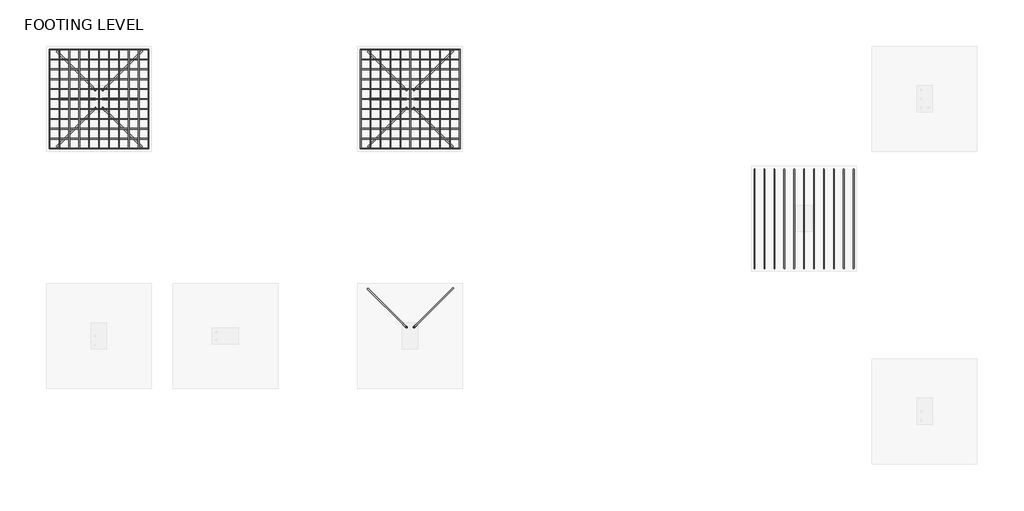
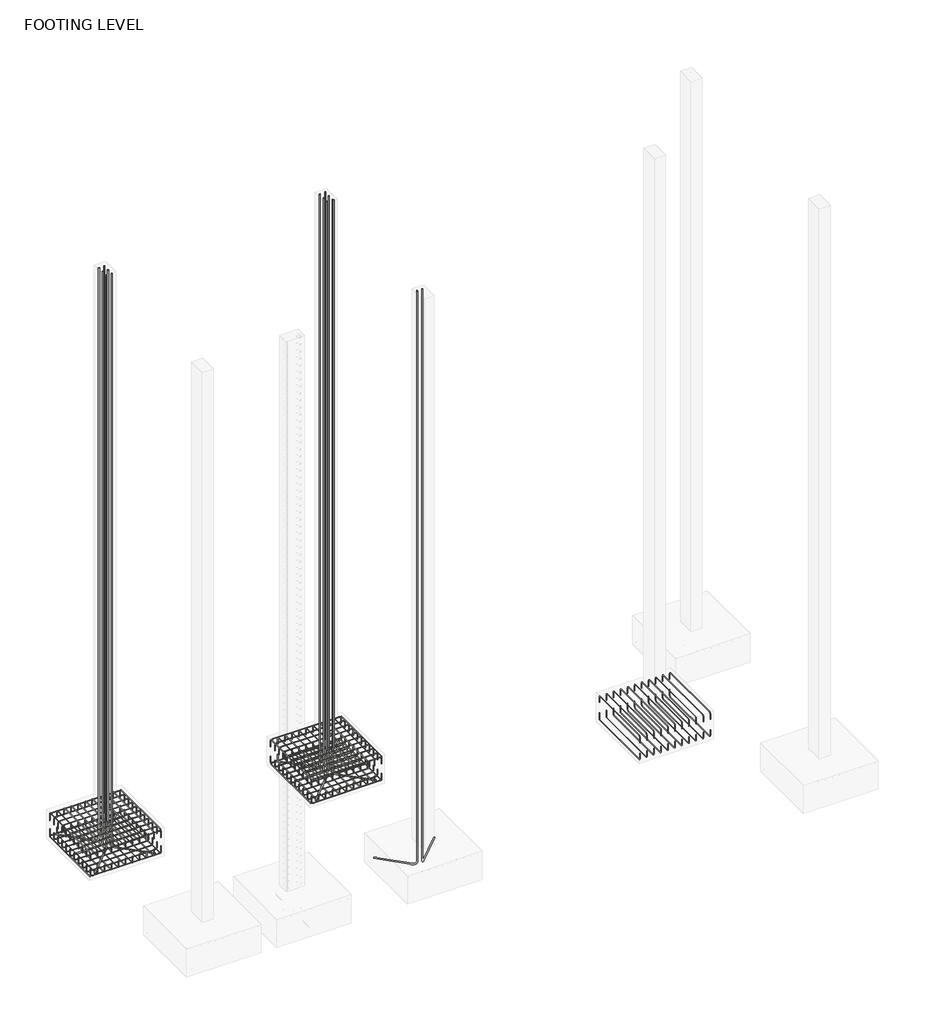
# One storey, part 9 of 10: 30 reinforcing bars.
"""IFC4 building model written with IfcOpenShell, lengths in millimetres."""

from ifc_helpers import new_model, si_unit, point, frame, origin, place, context, project, spatial, polyline, circle_curve, trimmed, segment, composite_curve, source, transform, mapped, element, save
from ifc_brep_helpers import swept_disk

model = new_model("IFC4")

# Units and contexts
model_context = context("Model", 3, world=origin())
ifc_project = project(units=[si_unit("LENGTHUNIT", "METRE", prefix="MILLI")], contexts=[model_context])

# Site, building, storey
site = spatial("IfcSite", under=ifc_project)
building = spatial("IfcBuilding", under=site)
storey = spatial("IfcBuildingStorey", under=building, Name="FOOTING LEVEL", Elevation=-1371.6)

# Reinforcing bars
placement = place(None, origin())
reinforcing_bar_shape = source(origin(), model_context, "Body", "SolidModel", [
    swept_disk(composite_curve([segment(polyline([(-9478.6043223, 13953.4953802, -1562.1), (-9478.6043223, 13953.4953802, -1447.8)]), True, "CONTINUOUS"), segment(trimmed(circle_curve(frame((-9478.6043223, 13920.1578802, -1447.8), z_axis=(1.0, 0.0, 0.0), x_axis=(0.0, 33.337499999999636, 0.0)), 33.3375), [point((-9478.6043223, 13953.4953802, -1447.8))], [point((-9478.6043223, 13920.1578802, -1414.4625))], True, "CARTESIAN"), True, "CONTINUOUS"), segment(polyline([(-9478.6043223, 13920.1578802, -1414.4625), (-9478.6043223, 12548.5578802, -1414.4625)]), True, "CONTINUOUS"), segment(trimmed(circle_curve(frame((-9478.6043223, 12548.5578802, -1447.8), z_axis=(1.0, 0.0, 0.0), x_axis=(0.0, 0.0, 33.337499999999864)), 33.3375), [point((-9478.6043223, 12548.5578802, -1414.4625))], [point((-9478.6043223, 12515.2203802, -1447.8))], True, "CARTESIAN"), True, "CONTINUOUS"), segment(polyline([(-9478.6043223, 12515.2203802, -1447.8), (-9478.6043223, 12515.2203802, -1562.1)]), True, "CONTINUOUS")], self_intersect=False), 4.7625),
])
element("IfcReinforcingBar", 1, at=placement, inside=storey, context=model_context, shape_type="MappedRepresentation", body=[
    mapped(reinforcing_bar_shape, transform((0.0, 0.0, 0.0), x_axis=(1.0, 0.0, 0.0), y_axis=(0.0, 1.0, 0.0), z_axis=(0.0, 0.0, 1.0))),
    mapped(reinforcing_bar_shape, transform((-143.8275, 0.0, 0.0), x_axis=(1.0, 0.0, 0.0), y_axis=(0.0, 1.0, 0.0), z_axis=(0.0, 0.0, 1.0))),
    mapped(reinforcing_bar_shape, transform((-287.655, 0.0, 0.0), x_axis=(1.0, 0.0, 0.0), y_axis=(0.0, 1.0, 0.0), z_axis=(0.0, 0.0, 1.0))),
    mapped(reinforcing_bar_shape, transform((-431.4825, 0.0, 0.0), x_axis=(1.0, 0.0, 0.0), y_axis=(0.0, 1.0, 0.0), z_axis=(0.0, 0.0, 1.0))),
    mapped(reinforcing_bar_shape, transform((-575.31, 0.0, 0.0), x_axis=(1.0, 0.0, 0.0), y_axis=(0.0, 1.0, 0.0), z_axis=(0.0, 0.0, 1.0))),
    mapped(reinforcing_bar_shape, transform((-719.1375, 0.0, 0.0), x_axis=(1.0, 0.0, 0.0), y_axis=(0.0, 1.0, 0.0), z_axis=(0.0, 0.0, 1.0))),
    mapped(reinforcing_bar_shape, transform((-862.965, 0.0, 0.0), x_axis=(1.0, 0.0, 0.0), y_axis=(0.0, 1.0, 0.0), z_axis=(0.0, 0.0, 1.0))),
    mapped(reinforcing_bar_shape, transform((-1006.7925, 0.0, 0.0), x_axis=(1.0, 0.0, 0.0), y_axis=(0.0, 1.0, 0.0), z_axis=(0.0, 0.0, 1.0))),
    mapped(reinforcing_bar_shape, transform((-1150.62, 0.0, 0.0), x_axis=(1.0, 0.0, 0.0), y_axis=(0.0, 1.0, 0.0), z_axis=(0.0, 0.0, 1.0))),
    mapped(reinforcing_bar_shape, transform((-1294.4475, 0.0, 0.0), x_axis=(1.0, 0.0, 0.0), y_axis=(0.0, 1.0, 0.0), z_axis=(0.0, 0.0, 1.0))),
    mapped(reinforcing_bar_shape, transform((-1438.275, 0.0, 0.0), x_axis=(1.0, 0.0, 0.0), y_axis=(0.0, 1.0, 0.0), z_axis=(0.0, 0.0, 1.0))),
])
reinforcing_bar_2_shape = source(origin(), model_context, "Body", "SolidModel", [
    swept_disk(composite_curve([segment(polyline([(-9478.6043223, 12515.2203802, -1790.7), (-9478.6043223, 12515.2203802, -1905.0)]), True, "CONTINUOUS"), segment(trimmed(circle_curve(frame((-9478.6043223, 12548.5578802, -1905.0), z_axis=(1.0, 0.0, 0.0), x_axis=(0.0, -33.337499999999636, 0.0)), 33.3375), [point((-9478.6043223, 12515.2203802, -1905.0))], [point((-9478.6043223, 12548.5578802, -1938.3375))], True, "CARTESIAN"), True, "CONTINUOUS"), segment(polyline([(-9478.6043223, 12548.5578802, -1938.3375), (-9478.6043223, 13920.1578802, -1938.3375)]), True, "CONTINUOUS"), segment(trimmed(circle_curve(frame((-9478.6043223, 13920.1578802, -1905.0), z_axis=(1.0, 0.0, 0.0), x_axis=(0.0, 0.0, -33.33750000000009)), 33.3375), [point((-9478.6043223, 13920.1578802, -1938.3375))], [point((-9478.6043223, 13953.4953802, -1905.0))], True, "CARTESIAN"), True, "CONTINUOUS"), segment(polyline([(-9478.6043223, 13953.4953802, -1905.0), (-9478.6043223, 13953.4953802, -1790.7)]), True, "CONTINUOUS")], self_intersect=False), 4.7625),
])
element("IfcReinforcingBar", 2, at=placement, inside=storey, context=model_context, shape_type="MappedRepresentation", body=[
    mapped(reinforcing_bar_2_shape, transform((0.0, 0.0, 0.0), x_axis=(1.0, 0.0, 0.0), y_axis=(0.0, 1.0, 0.0), z_axis=(0.0, 0.0, 1.0))),
    mapped(reinforcing_bar_2_shape, transform((-143.8275, 0.0, 0.0), x_axis=(1.0, 0.0, 0.0), y_axis=(0.0, 1.0, 0.0), z_axis=(0.0, 0.0, 1.0))),
    mapped(reinforcing_bar_2_shape, transform((-287.655, 0.0, 0.0), x_axis=(1.0, 0.0, 0.0), y_axis=(0.0, 1.0, 0.0), z_axis=(0.0, 0.0, 1.0))),
    mapped(reinforcing_bar_2_shape, transform((-431.4825, 0.0, 0.0), x_axis=(1.0, 0.0, 0.0), y_axis=(0.0, 1.0, 0.0), z_axis=(0.0, 0.0, 1.0))),
    mapped(reinforcing_bar_2_shape, transform((-575.31, 0.0, 0.0), x_axis=(1.0, 0.0, 0.0), y_axis=(0.0, 1.0, 0.0), z_axis=(0.0, 0.0, 1.0))),
    mapped(reinforcing_bar_2_shape, transform((-719.1375, 0.0, 0.0), x_axis=(1.0, 0.0, 0.0), y_axis=(0.0, 1.0, 0.0), z_axis=(0.0, 0.0, 1.0))),
    mapped(reinforcing_bar_2_shape, transform((-862.965, 0.0, 0.0), x_axis=(1.0, 0.0, 0.0), y_axis=(0.0, 1.0, 0.0), z_axis=(0.0, 0.0, 1.0))),
    mapped(reinforcing_bar_2_shape, transform((-1006.7925, 0.0, 0.0), x_axis=(1.0, 0.0, 0.0), y_axis=(0.0, 1.0, 0.0), z_axis=(0.0, 0.0, 1.0))),
    mapped(reinforcing_bar_2_shape, transform((-1150.62, 0.0, 0.0), x_axis=(1.0, 0.0, 0.0), y_axis=(0.0, 1.0, 0.0), z_axis=(0.0, 0.0, 1.0))),
    mapped(reinforcing_bar_2_shape, transform((-1294.4475, 0.0, 0.0), x_axis=(1.0, 0.0, 0.0), y_axis=(0.0, 1.0, 0.0), z_axis=(0.0, 0.0, 1.0))),
    mapped(reinforcing_bar_2_shape, transform((-1438.275, 0.0, 0.0), x_axis=(1.0, 0.0, 0.0), y_axis=(0.0, 1.0, 0.0), z_axis=(0.0, 0.0, 1.0))),
])
reinforcing_bar_3_shape = source(origin(), model_context, "Body", "SolidModel", [
    swept_disk(composite_curve([segment(polyline([(-13993.4543223, 13953.4953802, -1562.1), (-13993.4543223, 13953.4953802, -1447.8)]), True, "CONTINUOUS"), segment(trimmed(circle_curve(frame((-13993.4543223, 13920.1578802, -1447.8), z_axis=(1.0, 0.0, 0.0), x_axis=(0.0, 33.337499999999636, 0.0)), 33.3375), [point((-13993.4543223, 13953.4953802, -1447.8))], [point((-13993.4543223, 13920.1578802, -1414.4625))], True, "CARTESIAN"), True, "CONTINUOUS"), segment(polyline([(-13993.4543223, 13920.1578802, -1414.4625), (-13993.4543223, 12548.5578802, -1414.4625)]), True, "CONTINUOUS"), segment(trimmed(circle_curve(frame((-13993.4543223, 12548.5578802, -1447.8), z_axis=(1.0, 0.0, 0.0), x_axis=(0.0, 0.0, 33.337499999999864)), 33.3375), [point((-13993.4543223, 12548.5578802, -1414.4625))], [point((-13993.4543223, 12515.2203802, -1447.8))], True, "CARTESIAN"), True, "CONTINUOUS"), segment(polyline([(-13993.4543223, 12515.2203802, -1447.8), (-13993.4543223, 12515.2203802, -1562.1)]), True, "CONTINUOUS")], self_intersect=False), 4.7625),
])
element("IfcReinforcingBar", 3, at=placement, inside=storey, context=model_context, shape_type="MappedRepresentation", body=[
    mapped(reinforcing_bar_3_shape, transform((0.0, 0.0, 0.0), x_axis=(1.0, 0.0, 0.0), y_axis=(0.0, 1.0, 0.0), z_axis=(0.0, 0.0, 1.0))),
    mapped(reinforcing_bar_3_shape, transform((-143.8275, 0.0, 0.0), x_axis=(1.0, 0.0, 0.0), y_axis=(0.0, 1.0, 0.0), z_axis=(0.0, 0.0, 1.0))),
    mapped(reinforcing_bar_3_shape, transform((-287.655, 0.0, 0.0), x_axis=(1.0, 0.0, 0.0), y_axis=(0.0, 1.0, 0.0), z_axis=(0.0, 0.0, 1.0))),
    mapped(reinforcing_bar_3_shape, transform((-431.4825, 0.0, 0.0), x_axis=(1.0, 0.0, 0.0), y_axis=(0.0, 1.0, 0.0), z_axis=(0.0, 0.0, 1.0))),
    mapped(reinforcing_bar_3_shape, transform((-575.31, 0.0, 0.0), x_axis=(1.0, 0.0, 0.0), y_axis=(0.0, 1.0, 0.0), z_axis=(0.0, 0.0, 1.0))),
    mapped(reinforcing_bar_3_shape, transform((-719.1375, 0.0, 0.0), x_axis=(1.0, 0.0, 0.0), y_axis=(0.0, 1.0, 0.0), z_axis=(0.0, 0.0, 1.0))),
    mapped(reinforcing_bar_3_shape, transform((-862.965, 0.0, 0.0), x_axis=(1.0, 0.0, 0.0), y_axis=(0.0, 1.0, 0.0), z_axis=(0.0, 0.0, 1.0))),
    mapped(reinforcing_bar_3_shape, transform((-1006.7925, 0.0, 0.0), x_axis=(1.0, 0.0, 0.0), y_axis=(0.0, 1.0, 0.0), z_axis=(0.0, 0.0, 1.0))),
    mapped(reinforcing_bar_3_shape, transform((-1150.62, 0.0, 0.0), x_axis=(1.0, 0.0, 0.0), y_axis=(0.0, 1.0, 0.0), z_axis=(0.0, 0.0, 1.0))),
    mapped(reinforcing_bar_3_shape, transform((-1294.4475, 0.0, 0.0), x_axis=(1.0, 0.0, 0.0), y_axis=(0.0, 1.0, 0.0), z_axis=(0.0, 0.0, 1.0))),
    mapped(reinforcing_bar_3_shape, transform((-1438.275, 0.0, 0.0), x_axis=(1.0, 0.0, 0.0), y_axis=(0.0, 1.0, 0.0), z_axis=(0.0, 0.0, 1.0))),
])
reinforcing_bar_4_shape = source(origin(), model_context, "Body", "SolidModel", [
    swept_disk(composite_curve([segment(polyline([(-13993.4543223, 12515.2203802, -1790.7), (-13993.4543223, 12515.2203802, -1905.0)]), True, "CONTINUOUS"), segment(trimmed(circle_curve(frame((-13993.4543223, 12548.5578802, -1905.0), z_axis=(1.0, 0.0, 0.0), x_axis=(0.0, -33.337499999999636, 0.0)), 33.3375), [point((-13993.4543223, 12515.2203802, -1905.0))], [point((-13993.4543223, 12548.5578802, -1938.3375))], True, "CARTESIAN"), True, "CONTINUOUS"), segment(polyline([(-13993.4543223, 12548.5578802, -1938.3375), (-13993.4543223, 13920.1578802, -1938.3375)]), True, "CONTINUOUS"), segment(trimmed(circle_curve(frame((-13993.4543223, 13920.1578802, -1905.0), z_axis=(1.0, 0.0, 0.0), x_axis=(0.0, 0.0, -33.33750000000009)), 33.3375), [point((-13993.4543223, 13920.1578802, -1938.3375))], [point((-13993.4543223, 13953.4953802, -1905.0))], True, "CARTESIAN"), True, "CONTINUOUS"), segment(polyline([(-13993.4543223, 13953.4953802, -1905.0), (-13993.4543223, 13953.4953802, -1790.7)]), True, "CONTINUOUS")], self_intersect=False), 4.7625),
])
element("IfcReinforcingBar", 4, at=placement, inside=storey, context=model_context, shape_type="MappedRepresentation", body=[
    mapped(reinforcing_bar_4_shape, transform((0.0, 0.0, 0.0), x_axis=(1.0, 0.0, 0.0), y_axis=(0.0, 1.0, 0.0), z_axis=(0.0, 0.0, 1.0))),
    mapped(reinforcing_bar_4_shape, transform((-143.8275, 0.0, 0.0), x_axis=(1.0, 0.0, 0.0), y_axis=(0.0, 1.0, 0.0), z_axis=(0.0, 0.0, 1.0))),
    mapped(reinforcing_bar_4_shape, transform((-287.655, 0.0, 0.0), x_axis=(1.0, 0.0, 0.0), y_axis=(0.0, 1.0, 0.0), z_axis=(0.0, 0.0, 1.0))),
    mapped(reinforcing_bar_4_shape, transform((-431.4825, 0.0, 0.0), x_axis=(1.0, 0.0, 0.0), y_axis=(0.0, 1.0, 0.0), z_axis=(0.0, 0.0, 1.0))),
    mapped(reinforcing_bar_4_shape, transform((-575.31, 0.0, 0.0), x_axis=(1.0, 0.0, 0.0), y_axis=(0.0, 1.0, 0.0), z_axis=(0.0, 0.0, 1.0))),
    mapped(reinforcing_bar_4_shape, transform((-719.1375, 0.0, 0.0), x_axis=(1.0, 0.0, 0.0), y_axis=(0.0, 1.0, 0.0), z_axis=(0.0, 0.0, 1.0))),
    mapped(reinforcing_bar_4_shape, transform((-862.965, 0.0, 0.0), x_axis=(1.0, 0.0, 0.0), y_axis=(0.0, 1.0, 0.0), z_axis=(0.0, 0.0, 1.0))),
    mapped(reinforcing_bar_4_shape, transform((-1006.7925, 0.0, 0.0), x_axis=(1.0, 0.0, 0.0), y_axis=(0.0, 1.0, 0.0), z_axis=(0.0, 0.0, 1.0))),
    mapped(reinforcing_bar_4_shape, transform((-1150.62, 0.0, 0.0), x_axis=(1.0, 0.0, 0.0), y_axis=(0.0, 1.0, 0.0), z_axis=(0.0, 0.0, 1.0))),
    mapped(reinforcing_bar_4_shape, transform((-1294.4475, 0.0, 0.0), x_axis=(1.0, 0.0, 0.0), y_axis=(0.0, 1.0, 0.0), z_axis=(0.0, 0.0, 1.0))),
    mapped(reinforcing_bar_4_shape, transform((-1438.275, 0.0, 0.0), x_axis=(1.0, 0.0, 0.0), y_axis=(0.0, 1.0, 0.0), z_axis=(0.0, 0.0, 1.0))),
])
reinforcing_bar_5_shape = source(origin(), model_context, "Body", "SolidModel", [
    swept_disk(composite_curve([segment(polyline([(-15431.7293223, 12515.2203802, -1770.864029), (-15431.7293223, 12515.2203802, -1885.164029)]), True, "CONTINUOUS"), segment(trimmed(circle_curve(frame((-15398.3918223, 12515.2203802, -1885.164029), z_axis=(0.0, -1.0, 0.0), x_axis=(-33.337499999999636, 0.0, 0.0)), 33.3375), [point((-15431.7293223, 12515.2203802, -1885.164029))], [point((-15398.3918223, 12515.2203802, -1918.501529))], True, "CARTESIAN"), True, "CONTINUOUS"), segment(polyline([(-15398.3918223, 12515.2203802, -1918.501529), (-14026.7918223, 12515.2203802, -1918.501529)]), True, "CONTINUOUS"), segment(trimmed(circle_curve(frame((-14026.7918223, 12515.2203802, -1885.164029), z_axis=(0.0, -1.0, 0.0), x_axis=(0.0, 0.0, -33.337499999999864)), 33.3375), [point((-14026.7918223, 12515.2203802, -1918.501529))], [point((-13993.4543223, 12515.2203802, -1885.164029))], True, "CARTESIAN"), True, "CONTINUOUS"), segment(polyline([(-13993.4543223, 12515.2203802, -1885.164029), (-13993.4543223, 12515.2203802, -1770.864029)]), True, "CONTINUOUS")], self_intersect=False), 4.7625),
])
element("IfcReinforcingBar", 5, at=placement, inside=storey, context=model_context, shape_type="MappedRepresentation", body=[
    mapped(reinforcing_bar_5_shape, transform((0.0, 0.0, 0.0), x_axis=(1.0, 0.0, 0.0), y_axis=(0.0, 1.0, 0.0), z_axis=(0.0, 0.0, 1.0))),
    mapped(reinforcing_bar_5_shape, transform((0.0, 143.8275, 0.0), x_axis=(1.0, 0.0, 0.0), y_axis=(0.0, 1.0, 0.0), z_axis=(0.0, 0.0, 1.0))),
    mapped(reinforcing_bar_5_shape, transform((0.0, 287.655, 0.0), x_axis=(1.0, 0.0, 0.0), y_axis=(0.0, 1.0, 0.0), z_axis=(0.0, 0.0, 1.0))),
    mapped(reinforcing_bar_5_shape, transform((0.0, 431.4825, 0.0), x_axis=(1.0, 0.0, 0.0), y_axis=(0.0, 1.0, 0.0), z_axis=(0.0, 0.0, 1.0))),
    mapped(reinforcing_bar_5_shape, transform((0.0, 575.31, 0.0), x_axis=(1.0, 0.0, 0.0), y_axis=(0.0, 1.0, 0.0), z_axis=(0.0, 0.0, 1.0))),
    mapped(reinforcing_bar_5_shape, transform((0.0, 719.1375, 0.0), x_axis=(1.0, 0.0, 0.0), y_axis=(0.0, 1.0, 0.0), z_axis=(0.0, 0.0, 1.0))),
    mapped(reinforcing_bar_5_shape, transform((0.0, 862.965, 0.0), x_axis=(1.0, 0.0, 0.0), y_axis=(0.0, 1.0, 0.0), z_axis=(0.0, 0.0, 1.0))),
    mapped(reinforcing_bar_5_shape, transform((0.0, 1006.7925, 0.0), x_axis=(1.0, 0.0, 0.0), y_axis=(0.0, 1.0, 0.0), z_axis=(0.0, 0.0, 1.0))),
    mapped(reinforcing_bar_5_shape, transform((0.0, 1150.62, 0.0), x_axis=(1.0, 0.0, 0.0), y_axis=(0.0, 1.0, 0.0), z_axis=(0.0, 0.0, 1.0))),
    mapped(reinforcing_bar_5_shape, transform((0.0, 1294.4475, 0.0), x_axis=(1.0, 0.0, 0.0), y_axis=(0.0, 1.0, 0.0), z_axis=(0.0, 0.0, 1.0))),
    mapped(reinforcing_bar_5_shape, transform((0.0, 1438.275, 0.0), x_axis=(1.0, 0.0, 0.0), y_axis=(0.0, 1.0, 0.0), z_axis=(0.0, 0.0, 1.0))),
])
reinforcing_bar_6_shape = source(origin(), model_context, "Body", "SolidModel", [
    swept_disk(composite_curve([segment(polyline([(-15431.7293223, 13953.4953802, -1586.5406765), (-15431.7293223, 13953.4953802, -1472.2406765)]), True, "CONTINUOUS"), segment(trimmed(circle_curve(frame((-15398.3918223, 13953.4953802, -1472.2406765), z_axis=(0.0, 1.0, 0.0), x_axis=(-33.337499999999636, 0.0, 0.0)), 33.3375), [point((-15431.7293223, 13953.4953802, -1472.2406765))], [point((-15398.3918223, 13953.4953802, -1438.9031765))], True, "CARTESIAN"), True, "CONTINUOUS"), segment(polyline([(-15398.3918223, 13953.4953802, -1438.9031765), (-14026.7918223, 13953.4953802, -1438.9031765)]), True, "CONTINUOUS"), segment(trimmed(circle_curve(frame((-14026.7918223, 13953.4953802, -1472.2406765), z_axis=(0.0, 1.0, 0.0), x_axis=(0.0, 0.0, 33.33750000000009)), 33.3375), [point((-14026.7918223, 13953.4953802, -1438.9031765))], [point((-13993.4543223, 13953.4953802, -1472.2406765))], True, "CARTESIAN"), True, "CONTINUOUS"), segment(polyline([(-13993.4543223, 13953.4953802, -1472.2406765), (-13993.4543223, 13953.4953802, -1586.5406765)]), True, "CONTINUOUS")], self_intersect=False), 4.7625),
])
element("IfcReinforcingBar", 6, at=placement, inside=storey, context=model_context, shape_type="MappedRepresentation", body=[
    mapped(reinforcing_bar_6_shape, transform((0.0, 0.0, 0.0), x_axis=(1.0, 0.0, 0.0), y_axis=(0.0, 1.0, 0.0), z_axis=(0.0, 0.0, 1.0))),
    mapped(reinforcing_bar_6_shape, transform((0.0, -143.8275, 0.0), x_axis=(1.0, 0.0, 0.0), y_axis=(0.0, 1.0, 0.0), z_axis=(0.0, 0.0, 1.0))),
    mapped(reinforcing_bar_6_shape, transform((0.0, -287.655, 0.0), x_axis=(1.0, 0.0, 0.0), y_axis=(0.0, 1.0, 0.0), z_axis=(0.0, 0.0, 1.0))),
    mapped(reinforcing_bar_6_shape, transform((0.0, -431.4825, 0.0), x_axis=(1.0, 0.0, 0.0), y_axis=(0.0, 1.0, 0.0), z_axis=(0.0, 0.0, 1.0))),
    mapped(reinforcing_bar_6_shape, transform((0.0, -575.31, 0.0), x_axis=(1.0, 0.0, 0.0), y_axis=(0.0, 1.0, 0.0), z_axis=(0.0, 0.0, 1.0))),
    mapped(reinforcing_bar_6_shape, transform((0.0, -719.1375, 0.0), x_axis=(1.0, 0.0, 0.0), y_axis=(0.0, 1.0, 0.0), z_axis=(0.0, 0.0, 1.0))),
    mapped(reinforcing_bar_6_shape, transform((0.0, -862.965, 0.0), x_axis=(1.0, 0.0, 0.0), y_axis=(0.0, 1.0, 0.0), z_axis=(0.0, 0.0, 1.0))),
    mapped(reinforcing_bar_6_shape, transform((0.0, -1006.7925, 0.0), x_axis=(1.0, 0.0, 0.0), y_axis=(0.0, 1.0, 0.0), z_axis=(0.0, 0.0, 1.0))),
    mapped(reinforcing_bar_6_shape, transform((0.0, -1150.62, 0.0), x_axis=(1.0, 0.0, 0.0), y_axis=(0.0, 1.0, 0.0), z_axis=(0.0, 0.0, 1.0))),
    mapped(reinforcing_bar_6_shape, transform((0.0, -1294.4475, 0.0), x_axis=(1.0, 0.0, 0.0), y_axis=(0.0, 1.0, 0.0), z_axis=(0.0, 0.0, 1.0))),
    mapped(reinforcing_bar_6_shape, transform((0.0, -1438.275, 0.0), x_axis=(1.0, 0.0, 0.0), y_axis=(0.0, 1.0, 0.0), z_axis=(0.0, 0.0, 1.0))),
])
reinforcing_bar_7_shape = source(origin(), model_context, "Body", "SolidModel", [
    swept_disk(composite_curve([segment(polyline([(-3763.6043223, 12216.291297, -1562.1), (-3763.6043223, 12216.291297, -1447.8)]), True, "CONTINUOUS"), segment(trimmed(circle_curve(frame((-3763.6043223, 12182.953797, -1447.8), z_axis=(1.0, 0.0, 0.0), x_axis=(0.0, 33.337499999999636, 0.0)), 33.3375), [point((-3763.6043223, 12216.291297, -1447.8))], [point((-3763.6043223, 12182.953797, -1414.4625))], True, "CARTESIAN"), True, "CONTINUOUS"), segment(polyline([(-3763.6043223, 12182.953797, -1414.4625), (-3763.6043223, 10811.353797, -1414.4625)]), True, "CONTINUOUS"), segment(trimmed(circle_curve(frame((-3763.6043223, 10811.353797, -1447.8), z_axis=(1.0, 0.0, 0.0), x_axis=(0.0, 0.0, 33.337499999999864)), 33.3375), [point((-3763.6043223, 10811.353797, -1414.4625))], [point((-3763.6043223, 10778.016297, -1447.8))], True, "CARTESIAN"), True, "CONTINUOUS"), segment(polyline([(-3763.6043223, 10778.016297, -1447.8), (-3763.6043223, 10778.016297, -1562.1)]), True, "CONTINUOUS")], self_intersect=False), 4.7625),
])
element("IfcReinforcingBar", 7, at=placement, inside=storey, context=model_context, shape_type="MappedRepresentation", body=[
    mapped(reinforcing_bar_7_shape, transform((0.0, 0.0, 0.0), x_axis=(1.0, 0.0, 0.0), y_axis=(0.0, 1.0, 0.0), z_axis=(0.0, 0.0, 1.0))),
    mapped(reinforcing_bar_7_shape, transform((-143.8275, 0.0, 0.0), x_axis=(1.0, 0.0, 0.0), y_axis=(0.0, 1.0, 0.0), z_axis=(0.0, 0.0, 1.0))),
    mapped(reinforcing_bar_7_shape, transform((-287.655, 0.0, 0.0), x_axis=(1.0, 0.0, 0.0), y_axis=(0.0, 1.0, 0.0), z_axis=(0.0, 0.0, 1.0))),
    mapped(reinforcing_bar_7_shape, transform((-431.4825, 0.0, 0.0), x_axis=(1.0, 0.0, 0.0), y_axis=(0.0, 1.0, 0.0), z_axis=(0.0, 0.0, 1.0))),
    mapped(reinforcing_bar_7_shape, transform((-575.31, 0.0, 0.0), x_axis=(1.0, 0.0, 0.0), y_axis=(0.0, 1.0, 0.0), z_axis=(0.0, 0.0, 1.0))),
    mapped(reinforcing_bar_7_shape, transform((-719.1375, 0.0, 0.0), x_axis=(1.0, 0.0, 0.0), y_axis=(0.0, 1.0, 0.0), z_axis=(0.0, 0.0, 1.0))),
    mapped(reinforcing_bar_7_shape, transform((-862.965, 0.0, 0.0), x_axis=(1.0, 0.0, 0.0), y_axis=(0.0, 1.0, 0.0), z_axis=(0.0, 0.0, 1.0))),
    mapped(reinforcing_bar_7_shape, transform((-1006.7925, 0.0, 0.0), x_axis=(1.0, 0.0, 0.0), y_axis=(0.0, 1.0, 0.0), z_axis=(0.0, 0.0, 1.0))),
    mapped(reinforcing_bar_7_shape, transform((-1150.62, 0.0, 0.0), x_axis=(1.0, 0.0, 0.0), y_axis=(0.0, 1.0, 0.0), z_axis=(0.0, 0.0, 1.0))),
    mapped(reinforcing_bar_7_shape, transform((-1294.4475, 0.0, 0.0), x_axis=(1.0, 0.0, 0.0), y_axis=(0.0, 1.0, 0.0), z_axis=(0.0, 0.0, 1.0))),
    mapped(reinforcing_bar_7_shape, transform((-1438.275, 0.0, 0.0), x_axis=(1.0, 0.0, 0.0), y_axis=(0.0, 1.0, 0.0), z_axis=(0.0, 0.0, 1.0))),
])
reinforcing_bar_8_shape = source(origin(), model_context, "Body", "SolidModel", [
    swept_disk(composite_curve([segment(polyline([(-3763.6043223, 10778.016297, -1790.7), (-3763.6043223, 10778.016297, -1905.0)]), True, "CONTINUOUS"), segment(trimmed(circle_curve(frame((-3763.6043223, 10811.353797, -1905.0), z_axis=(1.0, 0.0, 0.0), x_axis=(0.0, -33.337499999999636, 0.0)), 33.3375), [point((-3763.6043223, 10778.016297, -1905.0))], [point((-3763.6043223, 10811.353797, -1938.3375))], True, "CARTESIAN"), True, "CONTINUOUS"), segment(polyline([(-3763.6043223, 10811.353797, -1938.3375), (-3763.6043223, 12182.953797, -1938.3375)]), True, "CONTINUOUS"), segment(trimmed(circle_curve(frame((-3763.6043223, 12182.953797, -1905.0), z_axis=(1.0, 0.0, 0.0), x_axis=(0.0, 0.0, -33.33750000000009)), 33.3375), [point((-3763.6043223, 12182.953797, -1938.3375))], [point((-3763.6043223, 12216.291297, -1905.0))], True, "CARTESIAN"), True, "CONTINUOUS"), segment(polyline([(-3763.6043223, 12216.291297, -1905.0), (-3763.6043223, 12216.291297, -1790.7)]), True, "CONTINUOUS")], self_intersect=False), 4.7625),
])
element("IfcReinforcingBar", 8, at=placement, inside=storey, context=model_context, shape_type="MappedRepresentation", body=[
    mapped(reinforcing_bar_8_shape, transform((0.0, 0.0, 0.0), x_axis=(1.0, 0.0, 0.0), y_axis=(0.0, 1.0, 0.0), z_axis=(0.0, 0.0, 1.0))),
    mapped(reinforcing_bar_8_shape, transform((-143.8275, 0.0, 0.0), x_axis=(1.0, 0.0, 0.0), y_axis=(0.0, 1.0, 0.0), z_axis=(0.0, 0.0, 1.0))),
    mapped(reinforcing_bar_8_shape, transform((-287.655, 0.0, 0.0), x_axis=(1.0, 0.0, 0.0), y_axis=(0.0, 1.0, 0.0), z_axis=(0.0, 0.0, 1.0))),
    mapped(reinforcing_bar_8_shape, transform((-431.4825, 0.0, 0.0), x_axis=(1.0, 0.0, 0.0), y_axis=(0.0, 1.0, 0.0), z_axis=(0.0, 0.0, 1.0))),
    mapped(reinforcing_bar_8_shape, transform((-575.31, 0.0, 0.0), x_axis=(1.0, 0.0, 0.0), y_axis=(0.0, 1.0, 0.0), z_axis=(0.0, 0.0, 1.0))),
    mapped(reinforcing_bar_8_shape, transform((-719.1375, 0.0, 0.0), x_axis=(1.0, 0.0, 0.0), y_axis=(0.0, 1.0, 0.0), z_axis=(0.0, 0.0, 1.0))),
    mapped(reinforcing_bar_8_shape, transform((-862.965, 0.0, 0.0), x_axis=(1.0, 0.0, 0.0), y_axis=(0.0, 1.0, 0.0), z_axis=(0.0, 0.0, 1.0))),
    mapped(reinforcing_bar_8_shape, transform((-1006.7925, 0.0, 0.0), x_axis=(1.0, 0.0, 0.0), y_axis=(0.0, 1.0, 0.0), z_axis=(0.0, 0.0, 1.0))),
    mapped(reinforcing_bar_8_shape, transform((-1150.62, 0.0, 0.0), x_axis=(1.0, 0.0, 0.0), y_axis=(0.0, 1.0, 0.0), z_axis=(0.0, 0.0, 1.0))),
    mapped(reinforcing_bar_8_shape, transform((-1294.4475, 0.0, 0.0), x_axis=(1.0, 0.0, 0.0), y_axis=(0.0, 1.0, 0.0), z_axis=(0.0, 0.0, 1.0))),
    mapped(reinforcing_bar_8_shape, transform((-1438.275, 0.0, 0.0), x_axis=(1.0, 0.0, 0.0), y_axis=(0.0, 1.0, 0.0), z_axis=(0.0, 0.0, 1.0))),
])
element("IfcReinforcingBar", 9, at=placement, inside=storey, context=model_context, shape_type="SolidModel", body=[
    swept_disk(composite_curve([segment(polyline([(-14658.2316302, 13364.9180723, -1333.5), (-14658.2316302, 13364.9180723, 10477.5)]), True, "CONTINUOUS")], self_intersect=False), 9.525),
])
element("IfcReinforcingBar", 10, at=placement, inside=storey, context=model_context, shape_type="SolidModel", body=[
    swept_disk(composite_curve([segment(polyline([(-14766.9520144, 13103.7976881, -1333.5), (-14766.9520144, 13103.7976881, 10477.5)]), True, "CONTINUOUS")], self_intersect=False), 9.525),
])
element("IfcReinforcingBar", 11, at=placement, inside=storey, context=model_context, shape_type="SolidModel", body=[
    swept_disk(composite_curve([segment(polyline([(-14658.2316302, 13103.7976881, -1333.5), (-14658.2316302, 13103.7976881, 10477.5)]), True, "CONTINUOUS")], self_intersect=False), 9.525),
])
element("IfcReinforcingBar", 12, at=placement, inside=storey, context=model_context, shape_type="SolidModel", body=[
    swept_disk(composite_curve([segment(polyline([(-15328.6277703, 13926.5938282, -1910.4342608), (-14814.0983591, 13412.0644169, -1910.4342608)]), True, "CONTINUOUS"), segment(trimmed(circle_curve(frame((-14814.0983591, 13412.0644169, -1843.7592608), z_axis=(-0.7071067811865736, -0.7071067811865216, 0.0), x_axis=(0.0, 0.0, -66.67499999999995)), 66.675), [point((-14814.0983591, 13412.0644169, -1910.4342608))], [point((-14766.9520144, 13364.9180723, -1843.7592608))], True, "CARTESIAN"), True, "CONTINUOUS"), segment(polyline([(-14766.9520144, 13364.9180723, -1843.7592608), (-14766.9520144, 13364.9180723, 10477.5)]), True, "CONTINUOUS")], self_intersect=False), 9.525),
])
element("IfcReinforcingBar", 13, at=placement, inside=storey, context=model_context, shape_type="SolidModel", body=[
    swept_disk(composite_curve([segment(polyline([(-14088.5374965, 13934.612206, -1910.4342608), (-14611.0852856, 13412.0644169, -1910.4342608)]), True, "CONTINUOUS"), segment(trimmed(circle_curve(frame((-14611.0852856, 13412.0644169, -1843.7592608), z_axis=(-0.7071067811865712, 0.7071067811865238, 0.0), x_axis=(0.0, 0.0, -66.67499999999995)), 66.675), [point((-14611.0852856, 13412.0644169, -1910.4342608))], [point((-14658.2316302, 13364.9180723, -1843.7592608))], True, "CARTESIAN"), True, "CONTINUOUS"), segment(polyline([(-14658.2316302, 13364.9180723, -1843.7592608), (-14658.2316302, 13364.9180723, 10477.5)]), True, "CONTINUOUS")], self_intersect=False), 9.525),
])
element("IfcReinforcingBar", 14, at=placement, inside=storey, context=model_context, shape_type="SolidModel", body=[
    swept_disk(composite_curve([segment(polyline([(-15325.6711349, 12545.0785676, -1910.4342608), (-14814.0983591, 13056.6513434, -1910.4342608)]), True, "CONTINUOUS"), segment(trimmed(circle_curve(frame((-14814.0983591, 13056.6513434, -1843.7592608), z_axis=(0.707106781186576, -0.7071067811865192, 0.0), x_axis=(0.0, 0.0, -66.67499999999995)), 66.675), [point((-14814.0983591, 13056.6513434, -1910.4342608))], [point((-14766.9520144, 13103.7976881, -1843.7592608))], True, "CARTESIAN"), True, "CONTINUOUS"), segment(polyline([(-14766.9520144, 13103.7976881, -1843.7592608), (-14766.9520144, 13103.7976881, 10477.5)]), True, "CONTINUOUS")], self_intersect=False), 9.525),
])
element("IfcReinforcingBar", 15, at=placement, inside=storey, context=model_context, shape_type="SolidModel", body=[
    swept_disk(composite_curve([segment(polyline([(-14094.0528099, 12539.6188678, -1910.4342608), (-14611.0852856, 13056.6513434, -1910.4342608)]), True, "CONTINUOUS"), segment(trimmed(circle_curve(frame((-14611.0852856, 13056.6513434, -1843.7592608), z_axis=(0.7071067811865689, 0.7071067811865261, 0.0), x_axis=(0.0, 0.0, -66.67499999999995)), 66.675), [point((-14611.0852856, 13056.6513434, -1910.4342608))], [point((-14658.2316302, 13103.7976881, -1843.7592608))], True, "CARTESIAN"), True, "CONTINUOUS"), segment(polyline([(-14658.2316302, 13103.7976881, -1843.7592608), (-14658.2316302, 13103.7976881, 10477.5)]), True, "CONTINUOUS")], self_intersect=False), 9.525),
])
element("IfcReinforcingBar", 16, at=placement, inside=storey, context=model_context, shape_type="SolidModel", body=[
    swept_disk(composite_curve([segment(polyline([(-15305.1818909, 13234.3578802, -1910.4342608), (-14833.6270144, 13234.3578802, -1910.4342608)]), True, "CONTINUOUS"), segment(trimmed(circle_curve(frame((-14833.6270144, 13234.3578802, -1843.7592608), z_axis=(0.0, -1.0, 0.0), x_axis=(0.0, 0.0, -66.67499999999995)), 66.675), [point((-14833.6270144, 13234.3578802, -1910.4342608))], [point((-14766.9520144, 13234.3578802, -1843.7592608))], True, "CARTESIAN"), True, "CONTINUOUS"), segment(polyline([(-14766.9520144, 13234.3578802, -1843.7592608), (-14766.9520144, 13234.3578802, 10477.5)]), True, "CONTINUOUS")], self_intersect=False), 9.525),
])
element("IfcReinforcingBar", 17, at=placement, inside=storey, context=model_context, shape_type="SolidModel", body=[
    swept_disk(composite_curve([segment(polyline([(-10130.6816302, 13377.6180723, -1346.2), (-10130.6816302, 13377.6180723, 10490.2)]), True, "CONTINUOUS")], self_intersect=False), 9.525),
])
element("IfcReinforcingBar", 18, at=placement, inside=storey, context=model_context, shape_type="SolidModel", body=[
    swept_disk(composite_curve([segment(polyline([(-10264.8020144, 13091.0976881, -1346.2), (-10264.8020144, 13091.0976881, 10490.2)]), True, "CONTINUOUS")], self_intersect=False), 9.525),
])
element("IfcReinforcingBar", 19, at=placement, inside=storey, context=model_context, shape_type="SolidModel", body=[
    swept_disk(composite_curve([segment(polyline([(-10130.6816302, 13091.0976881, -1346.2), (-10130.6816302, 13091.0976881, 10490.2)]), True, "CONTINUOUS")], self_intersect=False), 9.525),
])
element("IfcReinforcingBar", 20, at=placement, inside=storey, context=model_context, shape_type="SolidModel", body=[
    swept_disk(composite_curve([segment(polyline([(-10813.7777703, 13926.5938282, -1910.4342608), (-10299.2483591, 13412.0644169, -1910.4342608)]), True, "CONTINUOUS"), segment(trimmed(circle_curve(frame((-10299.2483591, 13412.0644169, -1843.7592608), z_axis=(-0.7071067811865736, -0.7071067811865216, 0.0), x_axis=(0.0, 0.0, -66.67499999999995)), 66.675), [point((-10299.2483591, 13412.0644169, -1910.4342608))], [point((-10252.1020144, 13364.9180723, -1843.7592608))], True, "CARTESIAN"), True, "CONTINUOUS"), segment(polyline([(-10252.1020144, 13364.9180723, -1843.7592608), (-10252.1020144, 13364.9180723, 10490.2)]), True, "CONTINUOUS")], self_intersect=False), 9.525),
])
element("IfcReinforcingBar", 21, at=placement, inside=storey, context=model_context, shape_type="SolidModel", body=[
    swept_disk(composite_curve([segment(polyline([(-9573.6874965, 13934.612206, -1910.4342608), (-10096.2352856, 13412.0644169, -1910.4342608)]), True, "CONTINUOUS"), segment(trimmed(circle_curve(frame((-10096.2352856, 13412.0644169, -1843.7592608), z_axis=(-0.7071067811865712, 0.7071067811865238, 0.0), x_axis=(0.0, 0.0, -66.67499999999995)), 66.675), [point((-10096.2352856, 13412.0644169, -1910.4342608))], [point((-10143.3816302, 13364.9180723, -1843.7592608))], True, "CARTESIAN"), True, "CONTINUOUS"), segment(polyline([(-10143.3816302, 13364.9180723, -1843.7592608), (-10143.3816302, 13364.9180723, 10490.2)]), True, "CONTINUOUS")], self_intersect=False), 9.525),
])
element("IfcReinforcingBar", 22, at=placement, inside=storey, context=model_context, shape_type="SolidModel", body=[
    swept_disk(composite_curve([segment(polyline([(-10810.8211349, 12545.0785676, -1910.4342608), (-10299.2483591, 13056.6513434, -1910.4342608)]), True, "CONTINUOUS"), segment(trimmed(circle_curve(frame((-10299.2483591, 13056.6513434, -1843.7592608), z_axis=(0.707106781186576, -0.7071067811865192, 0.0), x_axis=(0.0, 0.0, -66.67499999999995)), 66.675), [point((-10299.2483591, 13056.6513434, -1910.4342608))], [point((-10252.1020144, 13103.7976881, -1843.7592608))], True, "CARTESIAN"), True, "CONTINUOUS"), segment(polyline([(-10252.1020144, 13103.7976881, -1843.7592608), (-10252.1020144, 13103.7976881, 10490.2)]), True, "CONTINUOUS")], self_intersect=False), 9.525),
])
element("IfcReinforcingBar", 23, at=placement, inside=storey, context=model_context, shape_type="SolidModel", body=[
    swept_disk(composite_curve([segment(polyline([(-9579.2028099, 12539.6188678, -1910.4342608), (-10096.2352856, 13056.6513434, -1910.4342608)]), True, "CONTINUOUS"), segment(trimmed(circle_curve(frame((-10096.2352856, 13056.6513434, -1843.7592608), z_axis=(0.7071067811865689, 0.7071067811865261, 0.0), x_axis=(0.0, 0.0, -66.67499999999995)), 66.675), [point((-10096.2352856, 13056.6513434, -1910.4342608))], [point((-10143.3816302, 13103.7976881, -1843.7592608))], True, "CARTESIAN"), True, "CONTINUOUS"), segment(polyline([(-10143.3816302, 13103.7976881, -1843.7592608), (-10143.3816302, 13103.7976881, 10490.2)]), True, "CONTINUOUS")], self_intersect=False), 9.525),
])
element("IfcReinforcingBar", 24, at=placement, inside=storey, context=model_context, shape_type="SolidModel", body=[
    swept_disk(composite_curve([segment(polyline([(-10790.3318909, 13234.3578802, -1910.4342608), (-10318.7770144, 13234.3578802, -1910.4342608)]), True, "CONTINUOUS"), segment(trimmed(circle_curve(frame((-10318.7770144, 13234.3578802, -1843.7592608), z_axis=(0.0, -1.0, 0.0), x_axis=(0.0, 0.0, -66.67499999999995)), 66.675), [point((-10318.7770144, 13234.3578802, -1910.4342608))], [point((-10252.1020144, 13234.3578802, -1843.7592608))], True, "CARTESIAN"), True, "CONTINUOUS"), segment(polyline([(-10252.1020144, 13234.3578802, -1843.7592608), (-10252.1020144, 13234.3578802, 10490.2)]), True, "CONTINUOUS")], self_intersect=False), 9.525),
])
element("IfcReinforcingBar", 25, at=placement, inside=storey, context=model_context, shape_type="SolidModel", body=[
    swept_disk(composite_curve([segment(polyline([(-10813.7777703, 10484.8938282, -1910.4342608), (-10299.2483591, 9970.3644169, -1910.4342608)]), True, "CONTINUOUS"), segment(trimmed(circle_curve(frame((-10299.2483591, 9970.3644169, -1843.7592608), z_axis=(-0.7071067811865737, -0.7071067811865215, 0.0), x_axis=(0.0, 0.0, -66.67499999999995)), 66.675), [point((-10299.2483591, 9970.3644169, -1910.4342608))], [point((-10252.1020144, 9923.2180723, -1843.7592608))], True, "CARTESIAN"), True, "CONTINUOUS"), segment(polyline([(-10252.1020144, 9923.2180723, -1843.7592608), (-10252.1020144, 9923.2180723, 10490.2)]), True, "CONTINUOUS")], self_intersect=False), 9.525),
])
element("IfcReinforcingBar", 26, at=placement, inside=storey, context=model_context, shape_type="SolidModel", body=[
    swept_disk(composite_curve([segment(polyline([(-9573.6874965, 10492.912206, -1910.4342608), (-10096.2352856, 9970.3644169, -1910.4342608)]), True, "CONTINUOUS"), segment(trimmed(circle_curve(frame((-10096.2352856, 9970.3644169, -1843.7592608), z_axis=(-0.7071067811865711, 0.7071067811865239, 0.0), x_axis=(0.0, 0.0, -66.67499999999995)), 66.675), [point((-10096.2352856, 9970.3644169, -1910.4342608))], [point((-10143.3816302, 9923.2180723, -1843.7592608))], True, "CARTESIAN"), True, "CONTINUOUS"), segment(polyline([(-10143.3816302, 9923.2180723, -1843.7592608), (-10143.3816302, 9923.2180723, 10490.2)]), True, "CONTINUOUS")], self_intersect=False), 9.525),
])
element("IfcReinforcingBar", 27, at=placement, inside=storey, context=model_context, shape_type="SolidModel", body=[
    swept_disk(composite_curve([segment(polyline([(-9605.1517538, 13234.3578802, -1910.4342608), (-10076.7066302, 13234.3578802, -1910.4342608)]), True, "CONTINUOUS"), segment(trimmed(circle_curve(frame((-10076.7066302, 13234.3578802, -1843.7592608), z_axis=(0.0, 1.0, 0.0), x_axis=(0.0, 0.0, -66.67499999999995)), 66.675), [point((-10076.7066302, 13234.3578802, -1910.4342608))], [point((-10143.3816302, 13234.3578802, -1843.7592608))], True, "CARTESIAN"), True, "CONTINUOUS"), segment(polyline([(-10143.3816302, 13234.3578802, -1843.7592608), (-10143.3816302, 13234.3578802, 10490.2)]), True, "CONTINUOUS")], self_intersect=False), 9.525),
])
element("IfcReinforcingBar", 28, at=placement, inside=storey, context=model_context, shape_type="SolidModel", body=[
    swept_disk(composite_curve([segment(polyline([(-14120.0017538, 13234.3578802, -1910.4342608), (-14591.5566302, 13234.3578802, -1910.4342608)]), True, "CONTINUOUS"), segment(trimmed(circle_curve(frame((-14591.5566302, 13234.3578802, -1843.7592608), z_axis=(0.0, 1.0, 0.0), x_axis=(0.0, 0.0, -66.67499999999995)), 66.675), [point((-14591.5566302, 13234.3578802, -1910.4342608))], [point((-14658.2316302, 13234.3578802, -1843.7592608))], True, "CARTESIAN"), True, "CONTINUOUS"), segment(polyline([(-14658.2316302, 13234.3578802, -1843.7592608), (-14658.2316302, 13234.3578802, 10477.5)]), True, "CONTINUOUS")], self_intersect=False), 9.525),
])
reinforcing_bar_9_shape = source(origin(), model_context, "Body", "SolidModel", [
    swept_disk(composite_curve([segment(polyline([(-10916.8793223, 12515.2203802, -1781.5411053), (-10916.8793223, 12515.2203802, -1895.8411053)]), True, "CONTINUOUS"), segment(trimmed(circle_curve(frame((-10883.5418223, 12515.2203802, -1895.8411053), z_axis=(0.0, -1.0, 0.0), x_axis=(-33.337499999999636, 0.0, 0.0)), 33.3375), [point((-10916.8793223, 12515.2203802, -1895.8411053))], [point((-10883.5418223, 12515.2203802, -1929.1786053))], True, "CARTESIAN"), True, "CONTINUOUS"), segment(polyline([(-10883.5418223, 12515.2203802, -1929.1786053), (-9511.9418223, 12515.2203802, -1929.1786053)]), True, "CONTINUOUS"), segment(trimmed(circle_curve(frame((-9511.9418223, 12515.2203802, -1895.8411053), z_axis=(0.0, -1.0, 0.0), x_axis=(0.0, 0.0, -33.33750000000009)), 33.3375), [point((-9511.9418223, 12515.2203802, -1929.1786053))], [point((-9478.6043223, 12515.2203802, -1895.8411053))], True, "CARTESIAN"), True, "CONTINUOUS"), segment(polyline([(-9478.6043223, 12515.2203802, -1895.8411053), (-9478.6043223, 12515.2203802, -1781.5411053)]), True, "CONTINUOUS")], self_intersect=False), 4.7625),
])
element("IfcReinforcingBar", 29, at=placement, inside=storey, context=model_context, shape_type="MappedRepresentation", body=[
    mapped(reinforcing_bar_9_shape, transform((0.0, 0.0, 0.0), x_axis=(1.0, 0.0, 0.0), y_axis=(0.0, 1.0, 0.0), z_axis=(0.0, 0.0, 1.0))),
    mapped(reinforcing_bar_9_shape, transform((0.0, 143.8275, 0.0), x_axis=(1.0, 0.0, 0.0), y_axis=(0.0, 1.0, 0.0), z_axis=(0.0, 0.0, 1.0))),
    mapped(reinforcing_bar_9_shape, transform((0.0, 287.655, 0.0), x_axis=(1.0, 0.0, 0.0), y_axis=(0.0, 1.0, 0.0), z_axis=(0.0, 0.0, 1.0))),
    mapped(reinforcing_bar_9_shape, transform((0.0, 431.4825, 0.0), x_axis=(1.0, 0.0, 0.0), y_axis=(0.0, 1.0, 0.0), z_axis=(0.0, 0.0, 1.0))),
    mapped(reinforcing_bar_9_shape, transform((0.0, 575.31, 0.0), x_axis=(1.0, 0.0, 0.0), y_axis=(0.0, 1.0, 0.0), z_axis=(0.0, 0.0, 1.0))),
    mapped(reinforcing_bar_9_shape, transform((0.0, 719.1375, 0.0), x_axis=(1.0, 0.0, 0.0), y_axis=(0.0, 1.0, 0.0), z_axis=(0.0, 0.0, 1.0))),
    mapped(reinforcing_bar_9_shape, transform((0.0, 862.965, 0.0), x_axis=(1.0, 0.0, 0.0), y_axis=(0.0, 1.0, 0.0), z_axis=(0.0, 0.0, 1.0))),
    mapped(reinforcing_bar_9_shape, transform((0.0, 1006.7925, 0.0), x_axis=(1.0, 0.0, 0.0), y_axis=(0.0, 1.0, 0.0), z_axis=(0.0, 0.0, 1.0))),
    mapped(reinforcing_bar_9_shape, transform((0.0, 1150.62, 0.0), x_axis=(1.0, 0.0, 0.0), y_axis=(0.0, 1.0, 0.0), z_axis=(0.0, 0.0, 1.0))),
    mapped(reinforcing_bar_9_shape, transform((0.0, 1294.4475, 0.0), x_axis=(1.0, 0.0, 0.0), y_axis=(0.0, 1.0, 0.0), z_axis=(0.0, 0.0, 1.0))),
    mapped(reinforcing_bar_9_shape, transform((0.0, 1438.275, 0.0), x_axis=(1.0, 0.0, 0.0), y_axis=(0.0, 1.0, 0.0), z_axis=(0.0, 0.0, 1.0))),
])
reinforcing_bar_10_shape = source(origin(), model_context, "Body", "SolidModel", [
    swept_disk(composite_curve([segment(polyline([(-10916.8793223, 13953.4953802, -1571.2325032), (-10916.8793223, 13953.4953802, -1456.9325032)]), True, "CONTINUOUS"), segment(trimmed(circle_curve(frame((-10883.5418223, 13953.4953802, -1456.9325032), z_axis=(0.0, 1.0, 0.0), x_axis=(-33.337499999999636, 0.0, 0.0)), 33.3375), [point((-10916.8793223, 13953.4953802, -1456.9325032))], [point((-10883.5418223, 13953.4953802, -1423.5950032))], True, "CARTESIAN"), True, "CONTINUOUS"), segment(polyline([(-10883.5418223, 13953.4953802, -1423.5950032), (-9511.9418223, 13953.4953802, -1423.5950032)]), True, "CONTINUOUS"), segment(trimmed(circle_curve(frame((-9511.9418223, 13953.4953802, -1456.9325032), z_axis=(0.0, 1.0, 0.0), x_axis=(0.0, 0.0, 33.337499999999864)), 33.3375), [point((-9511.9418223, 13953.4953802, -1423.5950032))], [point((-9478.6043223, 13953.4953802, -1456.9325032))], True, "CARTESIAN"), True, "CONTINUOUS"), segment(polyline([(-9478.6043223, 13953.4953802, -1456.9325032), (-9478.6043223, 13953.4953802, -1571.2325032)]), True, "CONTINUOUS")], self_intersect=False), 4.7625),
])
element("IfcReinforcingBar", 30, at=placement, inside=storey, context=model_context, shape_type="MappedRepresentation", body=[
    mapped(reinforcing_bar_10_shape, transform((0.0, 0.0, 0.0), x_axis=(1.0, 0.0, 0.0), y_axis=(0.0, 1.0, 0.0), z_axis=(0.0, 0.0, 1.0))),
    mapped(reinforcing_bar_10_shape, transform((0.0, -143.8275, 0.0), x_axis=(1.0, 0.0, 0.0), y_axis=(0.0, 1.0, 0.0), z_axis=(0.0, 0.0, 1.0))),
    mapped(reinforcing_bar_10_shape, transform((0.0, -287.655, 0.0), x_axis=(1.0, 0.0, 0.0), y_axis=(0.0, 1.0, 0.0), z_axis=(0.0, 0.0, 1.0))),
    mapped(reinforcing_bar_10_shape, transform((0.0, -431.4825, 0.0), x_axis=(1.0, 0.0, 0.0), y_axis=(0.0, 1.0, 0.0), z_axis=(0.0, 0.0, 1.0))),
    mapped(reinforcing_bar_10_shape, transform((0.0, -575.31, 0.0), x_axis=(1.0, 0.0, 0.0), y_axis=(0.0, 1.0, 0.0), z_axis=(0.0, 0.0, 1.0))),
    mapped(reinforcing_bar_10_shape, transform((0.0, -719.1375, 0.0), x_axis=(1.0, 0.0, 0.0), y_axis=(0.0, 1.0, 0.0), z_axis=(0.0, 0.0, 1.0))),
    mapped(reinforcing_bar_10_shape, transform((0.0, -862.965, 0.0), x_axis=(1.0, 0.0, 0.0), y_axis=(0.0, 1.0, 0.0), z_axis=(0.0, 0.0, 1.0))),
    mapped(reinforcing_bar_10_shape, transform((0.0, -1006.7925, 0.0), x_axis=(1.0, 0.0, 0.0), y_axis=(0.0, 1.0, 0.0), z_axis=(0.0, 0.0, 1.0))),
    mapped(reinforcing_bar_10_shape, transform((0.0, -1150.62, 0.0), x_axis=(1.0, 0.0, 0.0), y_axis=(0.0, 1.0, 0.0), z_axis=(0.0, 0.0, 1.0))),
    mapped(reinforcing_bar_10_shape, transform((0.0, -1294.4475, 0.0), x_axis=(1.0, 0.0, 0.0), y_axis=(0.0, 1.0, 0.0), z_axis=(0.0, 0.0, 1.0))),
    mapped(reinforcing_bar_10_shape, transform((0.0, -1438.275, 0.0), x_axis=(1.0, 0.0, 0.0), y_axis=(0.0, 1.0, 0.0), z_axis=(0.0, 0.0, 1.0))),
])

save(model, "model.ifc")

# Revit data of these elements
# Elements 1, 2, 3, 4, 5, 6, 7, 8, 9, 10, 11, 12, 13, 14, 15, 16, 17, 18, 19, 20, 21, 22, 23, 24, 25, 26, 27, 28, 29, 30 (IfcReinforcingBar)
#   Phase Created = New Construction
